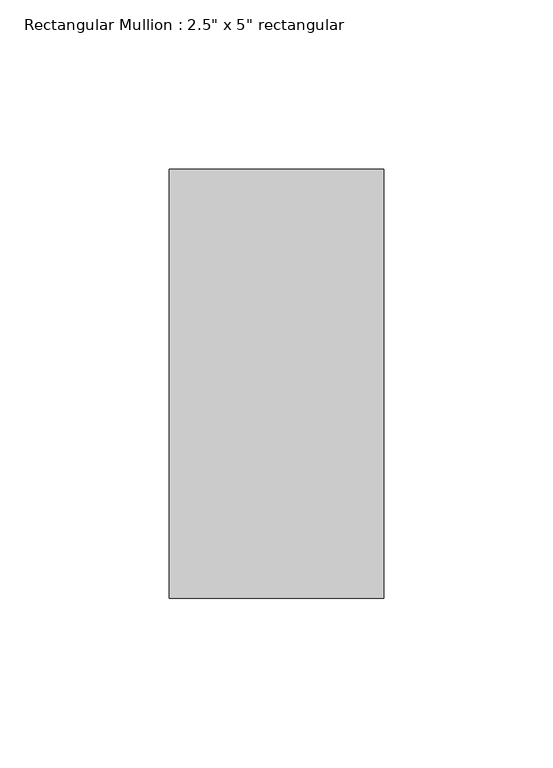
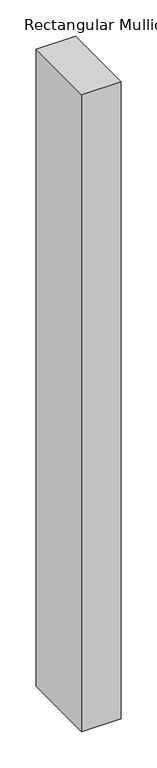
"""IFC4 building model written with IfcOpenShell, lengths in millimetres: member geometry."""

from ifc_helpers import new_model, si_unit, frame, origin, place, context, project, spatial, polyline, outline, extrude, source, transform, mapped, element, save


def member_74e81316(model_context):
    return source(origin(), model_context, "Body", "SweptSolid", [
        extrude(outline(polyline([(0.0, 63.5), (0.0, -63.5), (-63.5, -63.5), (-63.5, 63.5), (0.0, 63.5)])), frame((0.0, 0.0, -1079.5), z_axis=(0.0, 0.0, 1.0), x_axis=(1.0, 0.0, 0.0)), (0.0, 0.0, 1.0), 1079.5),
    ])


if __name__ == "__main__":
    model = new_model("IFC4")
    model_context = context("Model", 3, world=origin())
    ifc_project = project(units=[si_unit("LENGTHUNIT", "METRE", prefix="MILLI")], contexts=[model_context])
    site = spatial("IfcSite", under=ifc_project)
    building = spatial("IfcBuilding", under=site)
    placement = place(None, origin())
    member_shape = member_74e81316(model_context)
    element("IfcMember", 1, ObjectType="Rectangular Mullion : 2.5\" x 5\" rectangular", at=placement, inside=building, context=model_context, shape_type="MappedRepresentation", body=[
        mapped(member_shape, transform((0.0, 0.0, 0.0), x_axis=(1.0, 0.0, 0.0), y_axis=(0.0, 1.0, 0.0), z_axis=(0.0, 0.0, 1.0))),
    ])
    save(model, "model.ifc")

# Revit data of these elements
# Type "Rectangular Mullion : 2.5\" x 5\" rectangular"
#   built-in parameter 1007304 = 0.416667 (stored number, unit not read)
#   built-in parameter 1007301 = 0.104167 (stored number, unit not read)
#   built-in parameter 1007300 = 0.104167 (stored number, unit not read)
# Element 1 (IfcMember, "Rectangular Mullion : 2.5\" x 5\" rectangular")
#   Materials on its faces: "Aluminum"
# Materials
#   "Aluminum": class "Metal", colour RGB 247 247 247, transparency 0, Description = "Aluminum 6061", Cost = 0
